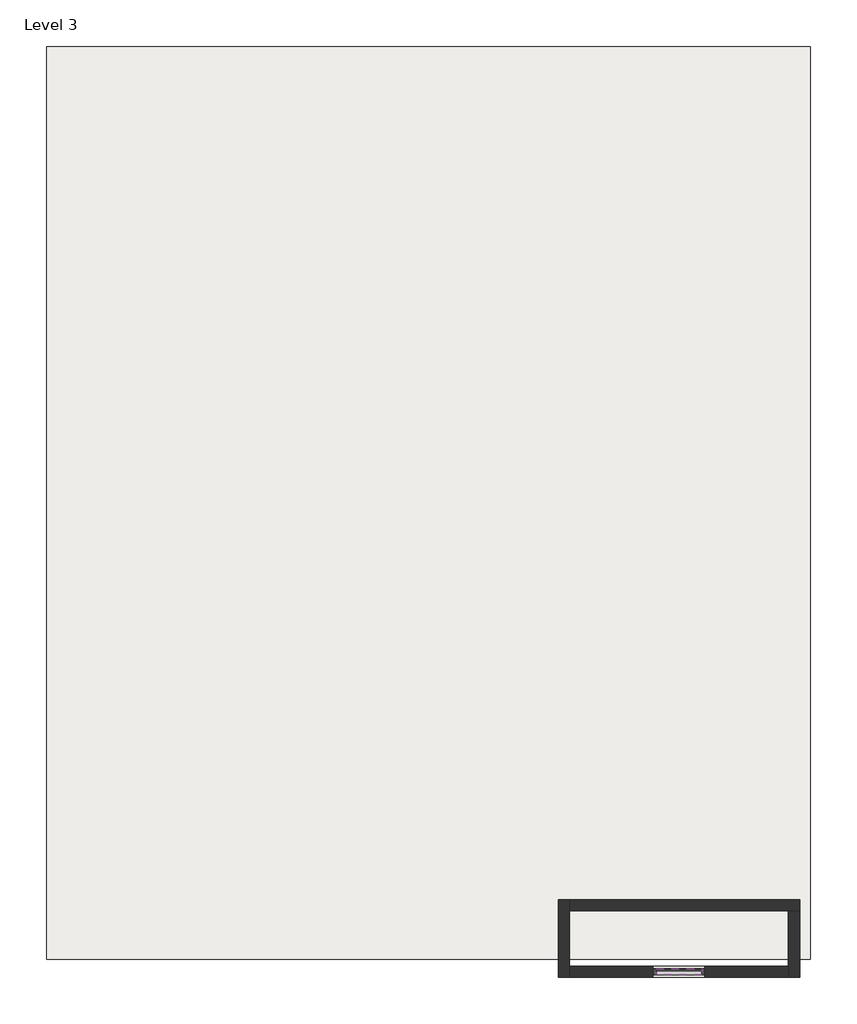
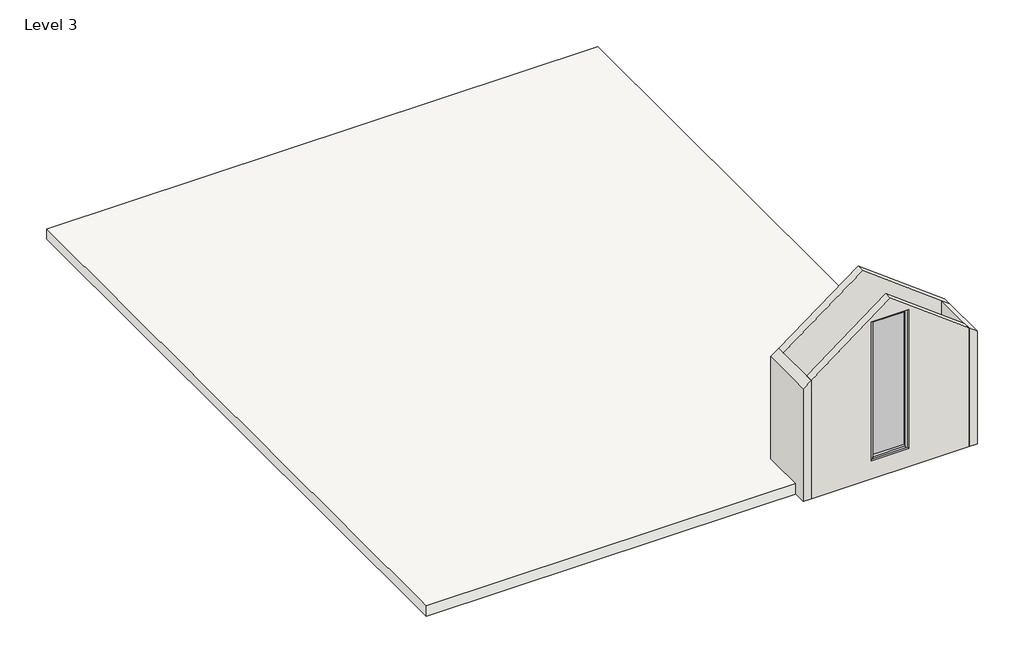
# One storey: 4 members, 4 walls, 1 plate, 1 roof.
"""IFC4 building model written with IfcOpenShell, lengths in millimetres."""

from ifc_helpers import new_model, si_unit, frame, origin, place, context, project, spatial, polyline, outline, extrude, faceted_brep, transform, mapped, element, save
from components import member_2dd2b658, member_d965e02f, system_panel_glazed_6cc658bf

model = new_model("IFC4")

# Units and contexts
model_context = context("Model", 3, world=origin())
ifc_project = project(units=[si_unit("LENGTHUNIT", "METRE", prefix="MILLI")], contexts=[model_context])

# Site, building, storey
site = spatial("IfcSite", under=ifc_project)
building = spatial("IfcBuilding", under=site)
storey = spatial("IfcBuildingStorey", under=building, Name="Level 3", Elevation=6096.0)

# Members
placement = place(None, origin())
member_shape = member_2dd2b658(model_context)
element("IfcMember", 1, ObjectType="Rectangular Mullion : 2.5\" x 5\" rectangular", at=placement, inside=storey, context=model_context, shape_type="MappedRepresentation", body=[
    mapped(member_shape, transform((-5623.7702714, -11844.7047424, 10826.0506676), x_axis=(0.0, 0.0, 1.0), y_axis=(0.0, -1.0, 0.0), z_axis=(1.0, 0.0, 0.0))),
])
element("IfcMember", 2, ObjectType="Rectangular Mullion : 2.5\" x 5\" rectangular", at=placement, inside=storey, context=model_context, shape_type="MappedRepresentation", body=[
    mapped(member_shape, transform((-6559.2418798, -11844.7047424, 6642.2571312), x_axis=(0.0, 0.0, -1.0), y_axis=(0.0, -1.0, 0.0), z_axis=(-1.0, 0.0, 0.0))),
])
member_2_shape = member_d965e02f(model_context)
element("IfcMember", 3, ObjectType="Rectangular Mullion : 2.5\" x 5\" rectangular", at=placement, inside=storey, context=model_context, shape_type="MappedRepresentation", body=[
    mapped(member_2_shape, transform((-6622.7418798, -11844.7047424, 10826.0506676), x_axis=(-1.0, 0.0, 0.0), y_axis=(0.0, -1.0, 0.0), z_axis=(0.0, 0.0, 1.0))),
])
element("IfcMember", 4, ObjectType="Rectangular Mullion : 2.5\" x 5\" rectangular", at=placement, inside=storey, context=model_context, shape_type="MappedRepresentation", body=[
    mapped(member_2_shape, transform((-5560.2702714, -11844.7047424, 6642.2571312), x_axis=(1.0, 0.0, 0.0), y_axis=(0.0, -1.0, 0.0), z_axis=(0.0, 0.0, -1.0))),
])

# Plate
system_panel_glazed_shape = system_panel_glazed_6cc658bf(model_context)
element("IfcPlate", 5, ObjectType="System Panel : Glazed", at=placement, inside=storey, context=model_context, shape_type="MappedRepresentation", body=[
    mapped(system_panel_glazed_shape, transform((-6091.5060756, -11844.7047424, 6705.7571312), x_axis=(1.0, 0.0, 0.0), y_axis=(0.0, 1.0, 0.0), z_axis=(0.0, 0.0, 1.0))),
])

# Roof
element("IfcRoof", 6, ObjectType="Generic - 12\"", at=placement, inside=storey, context=model_context, shape_type="SweptSolid", body=[
    extrude(outline(polyline([(-19085.7702714, 7157.4616097), (-3388.5702714, 7157.4616097), (-3388.5702714, -11587.7383903), (-19085.7702714, -11587.7383903), (-19085.7702714, 7157.4616097)])), frame((0.0, 0.0, 6096.0), z_axis=(0.0, 0.0, 1.0), x_axis=(1.0, 0.0, 0.0)), (0.0, 0.0, 1.0), 304.8),
])

# Walls
element("IfcWall", 7, ObjectType="9\"", at=placement, inside=storey, context=model_context, shape_type="Brep", body=[
    faceted_brep([(-8337.2418798, -11959.0047424, 6096.0), (-8337.2418798, -11730.4047424, 6096.0), (-8337.2418798, -10587.4047424, 6096.0), (-8337.2418798, -10358.8047424, 6096.0), (-8337.2418798, -10358.8047424, 9656.9556616), (-8337.2418798, -10587.4047424, 9656.9556616), (-8337.2418798, -11730.4047424, 9656.9556616), (-8337.2418798, -11959.0047424, 9656.9556616), (-8565.8418798, -11959.0047424, 6096.0), (-8565.8418798, -11959.0047424, 9485.5056616), (-8565.8418798, -10358.8047424, 9485.5056616), (-8565.8418798, -10358.8047424, 6096.0)], [[[0, 1, 2, 3, 4, 5, 6, 7]], [[8, 9, 10, 11]], [[3, 2, 1, 0, 8, 11]], [[4, 3, 11, 10]], [[0, 7, 9, 8]], [[7, 6, 5, 4, 10, 9]]]),
])
element("IfcWall", 8, ObjectType="9\"", at=placement, inside=storey, context=model_context, shape_type="Brep", body=[
    faceted_brep([(-8337.2418798, -10587.4047424, 6096.0), (-3841.4418798, -10587.4047424, 6096.0), (-3612.8418798, -10587.4047424, 6096.0), (-3612.8418798, -10587.4047424, 9497.5229256), (-3841.4418798, -10587.4047424, 9668.9729256), (-6081.3303705, -10587.4047424, 11348.8892936), (-8337.2418798, -10587.4047424, 9656.9556616), (-8337.2418798, -10358.8047424, 6096.0), (-8337.2418798, -10358.8047424, 9656.9556616), (-6081.3303705, -10358.8047424, 11348.8892936), (-3612.8418798, -10358.8047424, 9497.5229256), (-3612.8418798, -10358.8047424, 6096.0)], [[[0, 1, 2, 3, 4, 5, 6]], [[7, 8, 9, 10, 11]], [[2, 1, 0, 7, 11]], [[0, 6, 8, 7]], [[3, 2, 11, 10]], [[6, 5, 9, 8]], [[5, 4, 3, 10, 9]]]),
])
element("IfcWall", 9, ObjectType="9\"", at=placement, inside=storey, context=model_context, shape_type="Brep", body=[
    faceted_brep([(-3841.4418798, -10587.4047424, 6096.0), (-3841.4418798, -11730.4047424, 6096.0), (-3841.4418798, -11959.0047424, 6096.0), (-3841.4418798, -11959.0047424, 9668.9729256), (-3841.4418798, -11730.4047424, 9668.9729256), (-3841.4418798, -10587.4047424, 9668.9729256), (-3612.8418798, -10587.4047424, 6096.0), (-3612.8418798, -10587.4047424, 9497.5229256), (-3612.8418798, -11959.0047424, 9497.5229256), (-3612.8418798, -11959.0047424, 6096.0)], [[[0, 1, 2, 3, 4, 5]], [[6, 7, 8, 9]], [[2, 1, 0, 6, 9]], [[0, 5, 7, 6]], [[3, 2, 9, 8]], [[5, 4, 3, 8, 7]]]),
])
element("IfcWall", 10, ObjectType="9\"", at=placement, inside=storey, context=model_context, shape_type="SweptSolid", body=[
    extrude(outline(polyline([(6096.0, -8337.2418798), (6096.0, -3841.4418798), (9668.9729256, -3841.4418798), (11348.8892936, -6081.3303705), (9656.9556616, -8337.2418798), (6096.0, -8337.2418798)]), holes=[polyline([(6642.2571312, -6622.7418798), (10826.0506676, -6622.7418798), (10826.0506676, -5560.2702714), (6642.2571312, -5560.2702714), (6642.2571312, -6622.7418798)])]), frame((0.0, -11959.0047424, 0.0), z_axis=(0.0, 1.0, 0.0), x_axis=(0.0, 0.0, 1.0)), (0.0, 0.0, 1.0), 228.6),
])

save(model, "model.ifc")

# Revit data of these elements
# Type "Rectangular Mullion : 2.5\" x 5\" rectangular"
#   built-in parameter 1007304 = 0.416667 (stored number, unit not read)
#   built-in parameter 1007301 = 0.104167 (stored number, unit not read)
#   built-in parameter 1007300 = 0.104167 (stored number, unit not read)
# Type "System Panel : Glazed"
#   Construction Type Id = "GSP4R"
#   Analytic Construction = "1/8 in Pilkington single glazing"
#   Visual Light Transmittance = 0.9
#   Solar Heat Gain Coefficient = 0.86
#   Heat Transfer Coefficient (U) = 1.18115 BTU/(h·ft²·°F)
#   Define Thermal Properties by = 1
# Type "Generic - 12\""
#   Assembly Code = "B1020"
#   Layers, outside or top first: 1' - 0" no material (function 1)
# Type "9\""
#   Assembly Code = "B2010"
#   Layers, outside or top first: 0' - 9" no material (function 1)
# Elements 1, 2, 3, 4 (IfcMember, "Rectangular Mullion : 2.5\" x 5\" rectangular")
#   Phase Created = New Construction
#   Materials on its faces: "Aluminum"
# Element 5 (IfcPlate, "System Panel : Glazed")
#   Phase Created = New Construction
#   Materials on its faces: "Glass"
# Element 6 (IfcRoof, "Generic - 12\"")
#   built-in parameter 1001705 = 21 (stored number, unit not read)
#   built-in parameter 1001710 = 33615
#   Phase Created = New Construction
#   Materials on its faces: "Default Roof"
# Elements 7, 8, 9, 10 (IfcWall, "9\"")
#   Top Offset = 0' - 0"
#   Base Offset = 0' - 0"
#   Unconnected Height = 10' - 0"
#   wall height = 10' - 0"
#   Phase Created = New Construction
#   Base Constraint = Level 3
#   Materials on its faces: "Default Wall"
# Materials
#   "Aluminum": class "Metal", colour RGB 247 247 247, transparency 0, Description = "Aluminum 6061", Cost = 0
#   "Glass": class "Glass", colour RGB 0 128 192, transparency 0.75, Description = "Soda Lime Glass", Cost = 0
#   "Default Roof": colour RGB 88 101 114, transparency 0, Cost = 0
#   "Default Wall": colour RGB 128 128 128, transparency 0, Cost = 0
